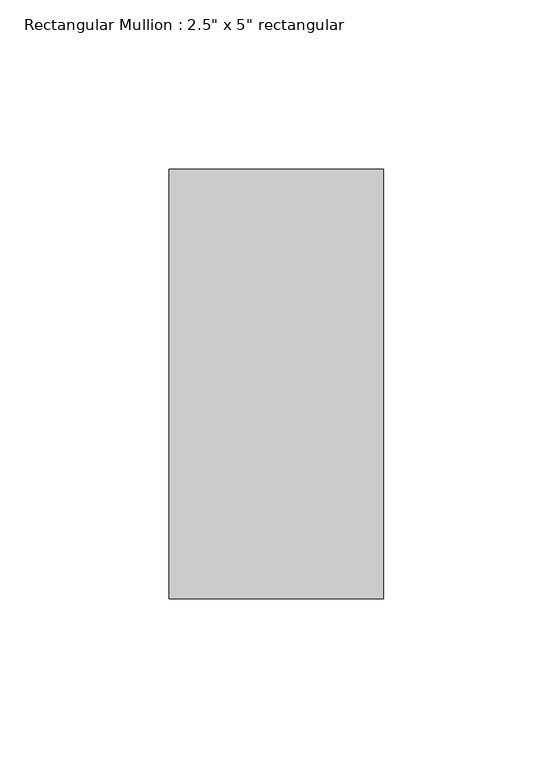
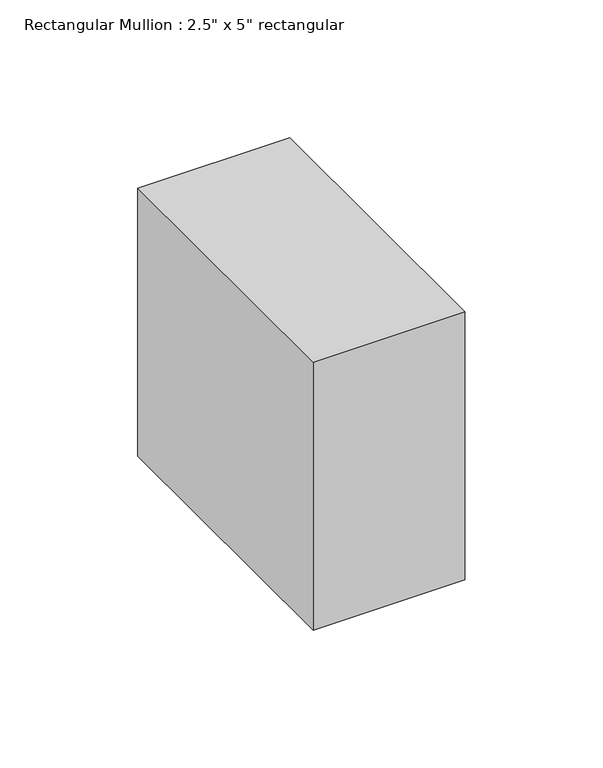
"""IFC4 building model written with IfcOpenShell, lengths in millimetres: member geometry."""

from ifc_helpers import new_model, si_unit, frame, origin, place, context, project, spatial, polyline, outline, extrude, source, transform, mapped, element, save


def member_6b3b9dad(model_context):
    return source(origin(), model_context, "Body", "SweptSolid", [
        extrude(outline(polyline([(0.0, 63.5), (0.0, -63.5), (-63.5, -63.5), (-63.5, 63.5), (0.0, 63.5)])), frame((0.0, 0.0, -118.5333333), z_axis=(0.0, 0.0, 1.0), x_axis=(1.0, 0.0, 0.0)), (0.0, 0.0, 1.0), 118.5333333),
    ])


if __name__ == "__main__":
    model = new_model("IFC4")
    model_context = context("Model", 3, world=origin())
    ifc_project = project(units=[si_unit("LENGTHUNIT", "METRE", prefix="MILLI")], contexts=[model_context])
    site = spatial("IfcSite", under=ifc_project)
    building = spatial("IfcBuilding", under=site)
    placement = place(None, origin())
    member_shape = member_6b3b9dad(model_context)
    element("IfcMember", 1, ObjectType="Rectangular Mullion : 2.5\" x 5\" rectangular", at=placement, inside=building, context=model_context, shape_type="MappedRepresentation", body=[
        mapped(member_shape, transform((0.0, 0.0, 0.0), x_axis=(1.0, 0.0, 0.0), y_axis=(0.0, 1.0, 0.0), z_axis=(0.0, 0.0, 1.0))),
    ])
    save(model, "model.ifc")

# Revit data of these elements
# Type "Rectangular Mullion : 2.5\" x 5\" rectangular"
#   built-in parameter 1007304 = 0.416667 (stored number, unit not read)
#   built-in parameter 1007301 = 0.104167 (stored number, unit not read)
#   built-in parameter 1007300 = 0.104167 (stored number, unit not read)
# Element 1 (IfcMember, "Rectangular Mullion : 2.5\" x 5\" rectangular")
#   Materials on its faces: "Aluminum"
# Materials
#   "Aluminum": class "Metal", colour RGB 247 247 247, transparency 0, Description = "Aluminum 6061", Cost = 0
